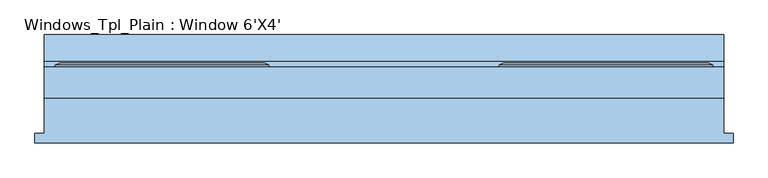
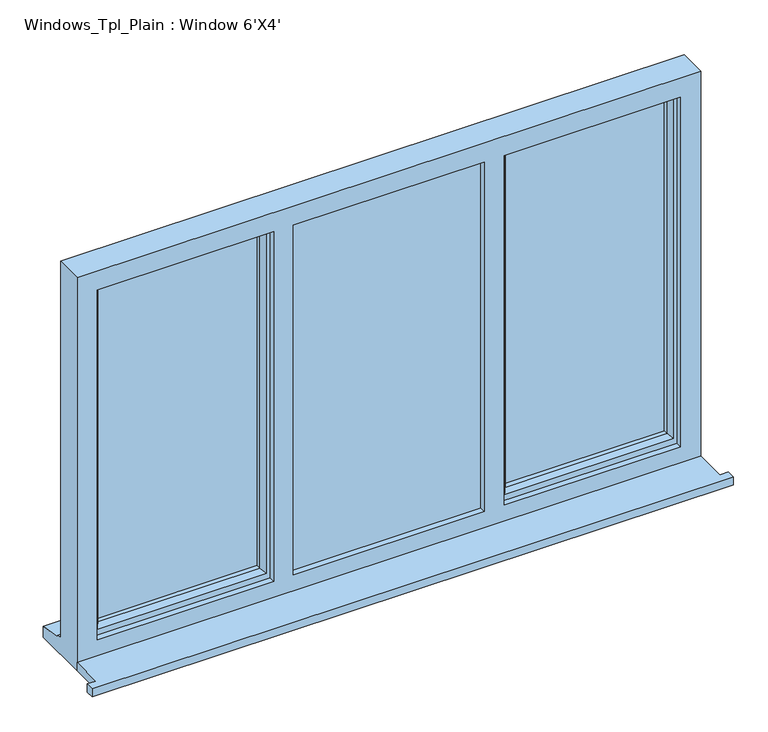
"""IFC4 building model written with IfcOpenShell, lengths in millimetres: window geometry, Windows_Tpl_Plain : Window 6'X4'."""

from ifc_helpers import new_model, si_unit, frame, origin, place, context, project, spatial, polyline, outline, extrude, faceted_brep, source, transform, mapped, element, save


def windows_tpl_plain_window_6_x4_c25596e0(model_context):
    return source(origin(), model_context, "Body", "SolidModel", [
        extrude(outline(polyline([(-1519.2, -130.8434322), (-1519.2, -105.8434322), (-1494.2, -105.8434322), (-1494.2, -10.2434322), (334.6, -10.2434322), (334.6, -105.8434322), (359.6, -105.8434322), (359.6, -130.8434322), (-1519.2, -130.8434322)])), frame((0.0, 0.0, 890.8), z_axis=(0.0, 0.0, 1.0), x_axis=(1.0, 0.0, 0.0)), (0.0, 0.0, 1.0), 25.0),
        faceted_brep([(-270.0, 72.7565678, 2080.0), (-270.0, 78.5300705, 2080.0), (-270.0, 78.5300705, 943.8), (-270.0, 72.7565678, 943.8), (-260.0, 7.7565678, 2070.0), (-260.0, 72.7565678, 2070.0), (-260.0, 72.7565678, 953.8), (-260.0, 7.7565678, 953.8), (-220.0, 22.2494677, 2030.0), (-230.1480377, 7.7565678, 2040.1480377), (-230.1480377, 7.7565678, 983.6519623), (-220.0, 22.2494677, 993.8), (-220.0, 36.7565678, 2030.0), (-220.0, 36.7565678, 993.8), (-230.0, 60.7565678, 2040.0), (-230.0, 36.7565678, 2040.0), (-230.0, 36.7565678, 983.8), (-230.0, 60.7565678, 983.8), (-220.0, 78.5300705, 2030.0), (-220.0, 60.7565678, 2030.0), (-220.0, 60.7565678, 993.8), (-220.0, 78.5300705, 993.8), (-237.4457548, 84.3035732, 2047.4457548), (-237.4457548, 84.3035732, 976.3542452), (-259.2153903, 84.3035732, 2069.2153903), (-259.2153903, 84.3035732, 954.5846097), (304.6, 78.5300705, 943.8), (304.6, 72.7565678, 943.8), (294.6, 72.7565678, 953.8), (294.6, 7.7565678, 953.8), (264.7480377, 7.7565678, 983.6519623), (254.6, 22.2494677, 993.8), (254.6, 36.7565678, 993.8), (264.6, 36.7565678, 983.8), (264.6, 60.7565678, 983.8), (254.6, 60.7565678, 993.8), (254.6, 78.5300705, 993.8), (272.0457548, 84.3035732, 976.3542452), (293.8153903, 84.3035732, 954.5846097), (304.6, 78.5300705, 2080.0), (304.6, 72.7565678, 2080.0), (294.6, 72.7565678, 2070.0), (294.6, 7.7565678, 2070.0), (264.7480377, 7.7565678, 2040.1480377), (254.6, 22.2494677, 2030.0), (254.6, 36.7565678, 2030.0), (264.6, 36.7565678, 2040.0), (264.6, 60.7565678, 2040.0), (254.6, 60.7565678, 2030.0), (254.6, 78.5300705, 2030.0), (272.0457548, 84.3035732, 2047.4457548), (293.8153903, 84.3035732, 2069.2153903)], [[[0, 1, 2, 3]], [[4, 5, 6, 7]], [[8, 9, 10, 11]], [[12, 8, 11, 13]], [[14, 15, 16, 17]], [[18, 19, 20, 21]], [[22, 18, 21, 23]], [[1, 24, 25, 2]], [[3, 2, 26, 27]], [[7, 6, 28, 29]], [[11, 10, 30, 31]], [[13, 11, 31, 32]], [[17, 16, 33, 34]], [[21, 20, 35, 36]], [[23, 21, 36, 37]], [[2, 25, 38, 26]], [[27, 26, 39, 40]], [[29, 28, 41, 42]], [[31, 30, 43, 44]], [[32, 31, 44, 45]], [[34, 33, 46, 47]], [[36, 35, 48, 49]], [[37, 36, 49, 50]], [[26, 38, 51, 39]], [[40, 39, 1, 0]], [[3, 27, 40, 0], [5, 41, 28, 6]], [[42, 41, 5, 4]], [[7, 29, 42, 4], [9, 43, 30, 10]], [[44, 43, 9, 8]], [[45, 44, 8, 12]], [[15, 46, 33, 16], [13, 32, 45, 12]], [[47, 46, 15, 14]], [[17, 34, 47, 14], [19, 48, 35, 20]], [[49, 48, 19, 18]], [[50, 49, 18, 22]], [[24, 51, 38, 25], [23, 37, 50, 22]], [[39, 51, 24, 1]]]),
        faceted_brep([(-889.6, 72.7565678, 2080.0), (-889.6, 78.5300705, 2080.0), (-1464.2, 78.5300705, 2080.0), (-1464.2, 72.7565678, 2080.0), (-899.6, 7.7565678, 2070.0), (-899.6, 72.7565678, 2070.0), (-1454.2, 72.7565678, 2070.0), (-1454.2, 7.7565678, 2070.0), (-939.6, 22.2494677, 2030.0), (-929.4519623, 7.7565678, 2040.1480377), (-1424.3480377, 7.7565678, 2040.1480377), (-1414.2, 22.2494677, 2030.0), (-939.6, 36.7565678, 2030.0), (-1414.2, 36.7565678, 2030.0), (-929.6, 60.7565678, 2040.0), (-929.6, 36.7565678, 2040.0), (-1424.2, 36.7565678, 2040.0), (-1424.2, 60.7565678, 2040.0), (-939.6, 78.5300705, 2030.0), (-939.6, 60.7565678, 2030.0), (-1414.2, 60.7565678, 2030.0), (-1414.2, 78.5300705, 2030.0), (-920.7854344, 84.3035732, 2048.8145656), (-1433.0145656, 84.3035732, 2048.8145656), (-901.2307806, 84.3035732, 2068.3692194), (-1452.5692194, 84.3035732, 2068.3692194), (-1464.2, 78.5300705, 943.8), (-1464.2, 72.7565678, 943.8), (-1454.2, 72.7565678, 953.8), (-1454.2, 7.7565678, 953.8), (-1424.3480377, 7.7565678, 983.6519623), (-1414.2, 22.2494677, 993.8), (-1414.2, 36.7565678, 993.8), (-1424.2, 36.7565678, 983.8), (-1424.2, 60.7565678, 983.8), (-1414.2, 60.7565678, 993.8), (-1414.2, 78.5300705, 993.8), (-1433.0145656, 84.3035732, 974.9854344), (-1452.5692194, 84.3035732, 955.4307806), (-889.6, 78.5300705, 943.8), (-889.6, 72.7565678, 943.8), (-899.6, 72.7565678, 953.8), (-899.6, 7.7565678, 953.8), (-929.4519623, 7.7565678, 983.6519623), (-939.6, 22.2494677, 993.8), (-939.6, 36.7565678, 993.8), (-929.6, 36.7565678, 983.8), (-929.6, 60.7565678, 983.8), (-939.6, 60.7565678, 993.8), (-939.6, 78.5300705, 993.8), (-920.7854344, 84.3035732, 974.9854344), (-901.2307806, 84.3035732, 955.4307806)], [[[0, 1, 2, 3]], [[4, 5, 6, 7]], [[8, 9, 10, 11]], [[12, 8, 11, 13]], [[14, 15, 16, 17]], [[18, 19, 20, 21]], [[22, 18, 21, 23]], [[1, 24, 25, 2]], [[3, 2, 26, 27]], [[7, 6, 28, 29]], [[11, 10, 30, 31]], [[13, 11, 31, 32]], [[17, 16, 33, 34]], [[21, 20, 35, 36]], [[23, 21, 36, 37]], [[2, 25, 38, 26]], [[27, 26, 39, 40]], [[0, 3, 27, 40], [41, 28, 6, 5]], [[29, 28, 41, 42]], [[4, 7, 29, 42], [43, 30, 10, 9]], [[31, 30, 43, 44]], [[32, 31, 44, 45]], [[46, 33, 16, 15], [12, 13, 32, 45]], [[34, 33, 46, 47]], [[14, 17, 34, 47], [48, 35, 20, 19]], [[36, 35, 48, 49]], [[37, 36, 49, 50]], [[51, 38, 25, 24], [22, 23, 37, 50]], [[26, 38, 51, 39]], [[40, 39, 1, 0]], [[42, 41, 5, 4]], [[44, 43, 9, 8]], [[45, 44, 8, 12]], [[47, 46, 15, 14]], [[49, 48, 19, 18]], [[50, 49, 18, 22]], [[39, 51, 24, 1]]]),
        faceted_brep([(334.6, -10.2434322, 2110.0), (-1494.2, -10.2434322, 2110.0), (-1494.2, -10.2434322, 890.8), (334.6, -10.2434322, 890.8), (274.6, -10.2434322, 2050.0), (274.6, -10.2434322, 965.8), (-242.0, -10.2434322, 965.8), (-242.0, -10.2434322, 2050.0), (-300.0, -10.2434322, 2050.0), (-300.0, -10.2434322, 965.8), (-859.6, -10.2434322, 965.8), (-859.6, -10.2434322, 2050.0), (-917.6, -10.2434322, 2050.0), (-917.6, -10.2434322, 965.8), (-1434.2, -10.2434322, 965.8), (-1434.2, -10.2434322, 2050.0), (-1494.2, 72.7565678, 2110.0), (-1494.2, 72.7565678, 941.8), (-1494.2, 87.7565678, 940.48767), (-1494.2, 87.7565678, 935.5449676), (-1494.2, 160.2565678, 924.6088847), (-1494.2, 160.2565678, 890.8), (334.6, 72.7565678, 2110.0), (334.6, 72.7565678, 941.8), (-1454.2, 72.7565678, 2070.0), (-1454.2, 72.7565678, 953.8), (-899.6, 72.7565678, 953.8), (-899.6, 72.7565678, 2070.0), (-859.6, 72.7565678, 2070.0), (-859.6, 72.7565678, 953.8), (-300.0, 72.7565678, 953.8), (-300.0, 72.7565678, 2070.0), (-260.0, 72.7565678, 2070.0), (-260.0, 72.7565678, 953.8), (294.6, 72.7565678, 953.8), (294.6, 72.7565678, 2070.0), (-1454.2, 7.7565678, 2070.0), (-1454.2, 7.7565678, 953.8), (-869.6, 7.7565678, 2070.0), (-290.0, 7.7565678, 2070.0), (-290.0, 7.7565678, 953.8), (-869.6, 7.7565678, 953.8), (-300.0, 7.7565678, 2050.0), (-859.6, 7.7565678, 2050.0), (-859.6, 7.7565678, 965.8), (-300.0, 7.7565678, 965.8), (-260.0, 7.7565678, 2070.0), (294.6, 7.7565678, 2070.0), (294.6, 7.7565678, 953.8), (-260.0, 7.7565678, 953.8), (274.6, 7.7565678, 2050.0), (-242.0, 7.7565678, 2050.0), (-242.0, 7.7565678, 965.8), (274.6, 7.7565678, 965.8), (-899.6, 7.7565678, 2070.0), (-899.6, 7.7565678, 953.8), (-917.6, 7.7565678, 2050.0), (-1434.2, 7.7565678, 2050.0), (-1434.2, 7.7565678, 965.8), (-917.6, 7.7565678, 965.8), (-859.6, 31.7565678, 2070.0), (-300.0, 31.7565678, 2070.0), (-290.0, 31.7565678, 2070.0), (-869.6, 31.7565678, 2070.0), (334.6, 160.2565678, 890.8), (334.6, 160.2565678, 924.6088847), (334.6, 87.7565678, 935.5449676), (334.6, 87.7565678, 940.48767), (-859.6, 31.7565678, 953.8), (-869.6, 31.7565678, 953.8), (-290.0, 31.7565678, 953.8), (-300.0, 31.7565678, 953.8)], [[[0, 1, 2, 3], [4, 5, 6, 7], [8, 9, 10, 11], [12, 13, 14, 15]], [[2, 1, 16, 17, 18, 19, 20, 21]], [[17, 16, 22, 23], [24, 25, 26, 27], [28, 29, 30, 31], [32, 33, 34, 35]], [[25, 24, 36, 37]], [[38, 39, 40, 41], [42, 43, 44, 45]], [[46, 47, 48, 49], [50, 51, 52, 53]], [[36, 54, 55, 37], [56, 57, 58, 59]], [[57, 15, 14, 58]], [[1, 0, 22, 16]], [[36, 24, 27, 54]], [[35, 47, 46, 32]], [[60, 28, 31, 61, 62, 39, 38, 63]], [[15, 57, 56, 12]], [[50, 4, 7, 51]], [[11, 43, 42, 8]], [[23, 22, 0, 3, 64, 65, 66, 67]], [[35, 34, 48, 47]], [[4, 50, 53, 5]], [[43, 11, 10, 44]], [[12, 56, 59, 13]], [[27, 26, 55, 54]], [[29, 28, 60, 68]], [[68, 60, 63, 69]], [[69, 63, 38, 41]], [[62, 70, 40, 39]], [[70, 62, 61, 71]], [[71, 61, 31, 30]], [[33, 32, 46, 49]], [[51, 7, 6, 52]], [[8, 42, 45, 9]], [[64, 3, 2, 21]], [[65, 64, 21, 20]], [[66, 65, 20, 19]], [[67, 66, 19, 18]], [[23, 67, 18, 17]], [[26, 25, 37, 55]], [[34, 33, 49, 48]], [[41, 40, 70, 71, 30, 29, 68, 69]], [[6, 5, 53, 52]], [[45, 44, 10, 9]], [[59, 58, 14, 13]]]),
        extrude(outline(polyline([(-929.6, 36.7565678), (-1424.2, 36.7565678), (-1424.2, 60.7565678), (-929.6, 60.7565678), (-929.6, 36.7565678)])), frame((0.0, 0.0, 983.8), z_axis=(0.0, 0.0, 1.0), x_axis=(1.0, 0.0, 0.0)), (0.0, 0.0, 1.0), 1056.2),
        extrude(outline(polyline([(-869.6, 31.7565678), (-290.0, 31.7565678), (-290.0, 7.7565678), (-869.6, 7.7565678), (-869.6, 31.7565678)])), frame((0.0, 0.0, 953.8), z_axis=(0.0, 0.0, 1.0), x_axis=(1.0, 0.0, 0.0)), (0.0, 0.0, 1.0), 1116.2),
        extrude(outline(polyline([(264.6, 36.7565678), (-230.0, 36.7565678), (-230.0, 60.7565678), (264.6, 60.7565678), (264.6, 36.7565678)])), frame((0.0, 0.0, 983.8), z_axis=(0.0, 0.0, 1.0), x_axis=(1.0, 0.0, 0.0)), (0.0, 0.0, 1.0), 1056.2),
    ])


if __name__ == "__main__":
    model = new_model("IFC4")
    model_context = context("Model", 3, world=origin())
    ifc_project = project(units=[si_unit("LENGTHUNIT", "METRE", prefix="MILLI")], contexts=[model_context])
    site = spatial("IfcSite", under=ifc_project)
    building = spatial("IfcBuilding", under=site)
    placement = place(None, origin())
    windows_tpl_plain_window_6_x4_shape = windows_tpl_plain_window_6_x4_c25596e0(model_context)
    element("IfcWindow", 1, ObjectType="Windows_Tpl_Plain : Window 6'X4'", at=placement, inside=building, context=model_context, shape_type="MappedRepresentation", body=[
        mapped(windows_tpl_plain_window_6_x4_shape, transform((0.0, 0.0, 0.0), x_axis=(1.0, 0.0, 0.0), y_axis=(0.0, 1.0, 0.0), z_axis=(0.0, 0.0, 1.0))),
    ])
    save(model, "model.ifc")

# Revit data of these elements
# Type "Windows_Tpl_Plain : Window 6'X4'"
#   Type Mark = "24"
#   Operation = "TriplePanelVertical"
#   Construction Type Id = "GSP4R"
#   Manufacturer = "Revit"
#   Keynote = "L10"
#   Analytic Construction = "1/8 in Pilkington single glazing"
#   Wrap Layers (Ext) from Ext = 0' - 4.03543"
#   Wrap Layers (Int) from Ext = 0' - 6.98819"
#   Window Board Projection = 0' - 0.98425"
#   Window Board Extension = 0' - 0.98425"
#   Visual Light Transmittance = 0.9
#   Solar Heat Gain Coefficient = 0.78
#   Rough Width = 6' - 0"
#   Rough Height = 4' - 0"
#   Height = 4' - 0"
#   Width = 6' - 0"
#   Heat Transfer Coefficient (U) = 0.6496 BTU/(h·ft²·°F)
#   Glazing Thickness = 0' - 0.94488"
#   FrameOffset - External = 0' - 1.9685"
#   Frame Depth = 0' - 2.55906"
#   Default Head Height = 6' - 11.07087"
#   Cill Depth = 0' - 3.44488"
#   Cavity Closer Width = 0' - 1.9685"
#   Cavity Closer Offset from Ext = 0' - 4.03543"
#   Cavity Closer Depth = 0' - 3.34646"
#   Vis - Cavity Closers = yes
#   Define Thermal Properties by = 1
#   Material Trim = Window Frame
#   Material Glass = Glass
#   Material Frame = Window Frame
#   Wall Closure = (empty or 0)
# Element 1 (IfcWindow, "Windows_Tpl_Plain : Window 6'X4'")
#   Materials on its faces: "Window Frame", "Glass"
# Materials
#   "Window Frame": colour RGB 249 249 249, transparency 0
#   "Glass": class "Glass", colour RGB 0 128 192, transparency 0.75, Description = "Soda Lime Glass", Cost = 0
